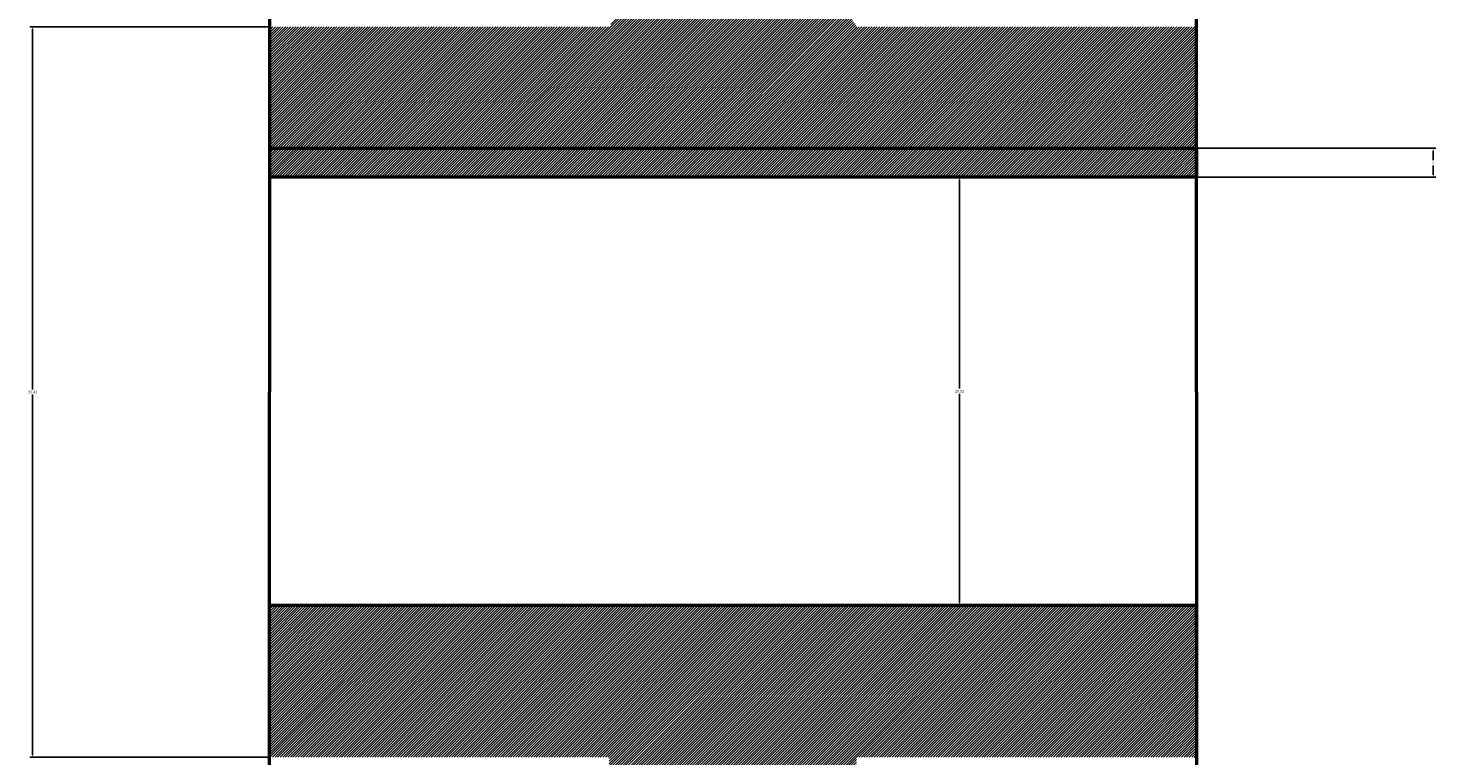
# Model space of a CAD drawing. Units: inches. Extents: x -99 to 284, y -92 to 134.
# Tile 14 of 16: x 187 to 284, y -11 to 39. Entities that reach past the tile are written whole.
import ezdxf

# ---------------------------------------------------------------- set-up
doc = ezdxf.new("R2010")
doc.units = ezdxf.units.IN
doc.header["$MEASUREMENT"] = 0
for name, color, linetype, lineweight in [('M-DIMS', 2, 'Continuous', 18), ('M-HATC', 8, 'Continuous', 18), ('M-OUTL', 7, 'Continuous', 50)]:
    doc.layers.add(name, color=color, linetype=linetype, lineweight=lineweight)
doc.styles.get("Standard").update_dxf_attribs({"font": 'arial.ttf'})
doc.dimstyles.get("Standard").update_dxf_attribs({"dimtxt": 0.18, "dimasz": 0.18, "dimexe": 0.18, "dimexo": 0.0625, "dimgap": 0.09, "dimtad": 0, "dimtih": 1, "dimtoh": 1, "dimdec": 4, "dimzin": 0, "dimdsep": 46, "dimtxsty": 'Standard', "dimcen": 0.09, "dimadec": 0, "dimazin": 0, "dimtfac": 1, "dimtdec": 4, "dimtofl": 0, "dimtmove": 0, "dimatfit": 3, "dimfxl": 1, "dimtolj": 1, "dimtzin": 0, "dimarcsym": 0})

# ---------------------------------------------------------------- blocks, each defined once
blk = doc.blocks.new('*D7')
at = {"layer": 'Defpoints', "color": 0, "transparency": 16777216}
for p in [(251.141, 28.552), (267.491, 28.552), (267.491, -0.969)]:
    blk.add_point(p, dxfattribs=at)
at = {"layer": 'M-DIMS', "color": 0, "lineweight": -2, "transparency": 16777216}
for p, q in [((267.429, 28.552), (250.961, 28.552)), ((251.141, 28.372), (251.141, 13.974)), ((251.141, -0.789), (251.141, 13.61)), ((267.429, -0.969), (250.961, -0.969))]:
    blk.add_line(p, q, dxfattribs=at)
at = {"layer": 'M-DIMS', "color": 0, "transparency": 16777216}
for points in [[(251.111, 28.372), (251.171, 28.372), (251.141, 28.552)], [(251.111, -0.789), (251.171, -0.789), (251.141, -0.969)]]:
    blk.add_solid(points, dxfattribs=at)
at = {"layer": 'M-DIMS', "color": 0, "transparency": 16777216, "insert": (251.141, 13.792), "char_height": 0.18, "attachment_point": 5}
blk.add_mtext('\\A1;29.52', dxfattribs=at)
blk = doc.blocks.new('*D12')
at = {"layer": 'Defpoints', "color": 0, "transparency": 16777216}
for p in [(187.141, 38.946), (203.491, 38.946), (203.491, -11.467)]:
    blk.add_point(p, dxfattribs=at)
at = {"layer": 'M-DIMS', "color": 0, "lineweight": -2, "transparency": 16777216}
for p, q in [((203.429, 38.946), (186.961, 38.946)), ((187.141, 38.766), (187.141, 13.922)), ((187.141, -11.287), (187.141, 13.558)), ((203.429, -11.467), (186.961, -11.467))]:
    blk.add_line(p, q, dxfattribs=at)
at = {"layer": 'M-DIMS', "color": 0, "transparency": 16777216}
for points in [[(187.111, 38.766), (187.171, 38.766), (187.141, 38.946)], [(187.111, -11.287), (187.171, -11.287), (187.141, -11.467)]]:
    blk.add_solid(points, dxfattribs=at)
at = {"layer": 'M-DIMS', "color": 0, "transparency": 16777216, "insert": (187.141, 13.74), "char_height": 0.18, "attachment_point": 5}
blk.add_mtext('\\A1;50.41', dxfattribs=at)
blk = doc.blocks.new('*D17')
at = {"layer": 'Defpoints', "color": 0, "transparency": 16777216}
for p in [(267.491, 30.552), (267.491, 28.552), (283.841, 28.552)]:
    blk.add_point(p, dxfattribs=at)
at = {"layer": 'M-DIMS', "color": 0, "lineweight": -2, "transparency": 16777216}
for p, q in [((267.554, 30.552), (284.021, 30.552)), ((283.841, 30.372), (283.841, 29.732)), ((283.841, 28.732), (283.841, 29.372)), ((267.554, 28.552), (284.021, 28.552))]:
    blk.add_line(p, q, dxfattribs=at)
at = {"layer": 'M-DIMS', "color": 0, "transparency": 16777216}
for points in [[(283.811, 30.372), (283.871, 30.372), (283.841, 30.552)], [(283.811, 28.732), (283.871, 28.732), (283.841, 28.552)]]:
    blk.add_solid(points, dxfattribs=at)
at = {"layer": 'M-DIMS', "color": 0, "transparency": 16777216, "insert": (283.841, 29.552), "char_height": 0.18, "attachment_point": 5}
blk.add_mtext('\\A1;2', dxfattribs=at)

msp = doc.modelspace()

# ---------------------------------------------------------------- hatches: boundary and pattern name
at = {"layer": 'M-HATC'}
h = msp.add_hatch(dxfattribs=at)
h.set_pattern_fill('ANSI31', color=256)
h.set_pattern_definition([(45, (-295.18303, 0), (-0.088388348, 0.088388348), [])])
h.paths.add_polyline_path([(235.9574, 102.7178), (260.4913, 101.5718), (260.4913, 98.6088), (240.4913, 97.7396, -1), (230.4913, 97.7396), (210.4913, 98.6088), (210.4913, 101.573), (235.4326, 102.7424), (235.4913, 102.7396, -0.0233428)])
h.paths.add_polyline_path([(226.9535, 38.946), (203.4913, 38.946), (203.4913, 30.5521), (267.4913, 30.5521), (267.4913, 38.946), (244.0291, 38.946, 0.5614625)])
h.paths.add_polyline_path([(267.4913, 30.5521), (203.4913, 30.5521), (203.4913, 28.5521), (267.4913, 28.5521)])
h.paths.add_polyline_path([(244.0291, -11.4667), (267.4913, -11.4667), (267.4913, -0.9688), (203.4913, -0.9688), (203.4913, -11.4667), (226.9535, -11.4667), (226.9535, -60.8393, -0.294228), (221.0875, -69.9448), (249.6222, -69.8159, -0.2860474), (244.0291, -60.8393)])
h.paths.add_polyline_path([(267.4913, -71.4338), (253.5949, -70.8299, -0.1036016), (249.6222, -69.8159), (221.0875, -69.9448, -0.095981), (217.3877, -70.8299), (203.4913, -71.4338), (203.4913, -73.7656), (235.2571, -75.2549, 0.0117126), (235.4913, -75.2604), (267.4913, -73.7656)])

# ---------------------------------------------------------------- linework, layer by layer
at = {"layer": 'M-OUTL'}
for p, q in [((203.4913, 101.2449), (203.4913, 13.7396)), ((267.4913, 13.7396), (267.4913, 101.2449)), ((267.4913, 13.7396), (267.4913, 38.7396)), ((203.4913, 30.5521), (267.4913, 30.5521)), ((267.4913, 30.5521), (267.4913, 28.5521)), ((267.4913, 28.5521), (203.4913, 28.5521)), ((203.4913, -73.7656), (203.4913, 13.7396)), ((267.4913, 13.7396), (267.4913, -73.7656)), ((267.4913, 13.7396), (267.4913, -11.2604)), ((203.4913, -0.9688), (267.4913, -0.9688)), ((267.4913, -3.0728), (267.4913, -1.0728))]:
    msp.add_line(p, q, dxfattribs=at)

# ---------------------------------------------------------------- dimensions: what is measured, and where the dimension line sits
at = {"layer": 'M-DIMS'}
for base, p1, p2, angle, override, picture, middle in [((187.1413, 38.946), (203.4913, -11.4667), (203.4913, 38.946), 90, {"dimdec": 2, "dimlfac": 1, "dimrnd": 0, "dimzin": 0, "dimdsep": 46, "dimlunit": 2}, '*D12', (187.1413, 13.7396)), ((283.8413, 28.5521), (267.4913, 30.5521), (267.4913, 28.5521), 270, {"dimdec": 0, "dimlfac": 1, "dimrnd": 0, "dimzin": 0, "dimdsep": 46, "dimlunit": 2}, '*D17', (283.8413, 29.5521)), ((251.1413, 28.5521), (267.4913, -0.9688), (267.4913, 28.5521), 90, {"dimdec": 2, "dimlfac": 1, "dimrnd": 0, "dimzin": 0, "dimdsep": 46, "dimlunit": 2}, '*D7', (251.1413, 13.7916))]:
    dim = msp.add_linear_dim(base=base, p1=p1, p2=p2, angle=angle, dimstyle='Standard', override=override, dxfattribs=at)
    dim.commit()
    dim.dimension.update_dxf_attribs({"geometry": picture, "text_midpoint": middle})

doc.saveas('drawing.dxf')
